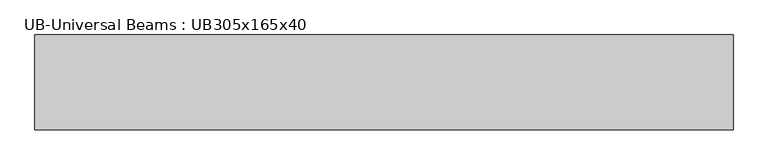
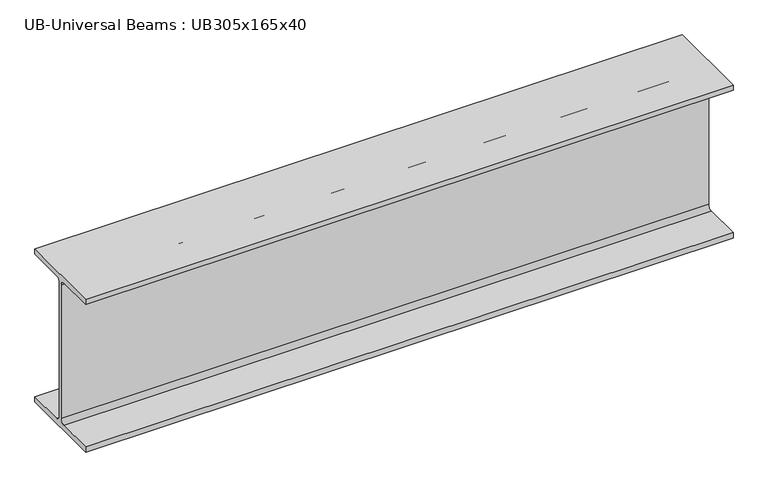
"""IFC4 building model written with IfcOpenShell, lengths in millimetres: beam geometry, UB-Universal Beams : UB305x165x40."""

from ifc_helpers import new_model, si_unit, point, frame, frame_2d, origin, place, context, project, spatial, polyline, circle_curve, trimmed, segment, composite_curve, outline, extrude, source, transform, mapped, element, save


def ub_universal_beams_ub305x165x40_babad7d3(model_context):
    return source(origin(), model_context, "Body", "SweptSolid", [
        extrude(outline(composite_curve([segment(polyline([(82.5, -141.5), (82.5, -151.7), (-82.5, -151.7), (-82.5, -141.5), (-11.9, -141.5)]), True, "CONTINUOUS"), segment(trimmed(circle_curve(frame_2d((-11.9, -132.6)), 8.9), [point((-11.9, -141.5))], [point((-3.0, -132.6))], True, "CARTESIAN"), True, "CONTINUOUS"), segment(polyline([(-3.0, -132.6), (-3.0, 132.6)]), True, "CONTINUOUS"), segment(trimmed(circle_curve(frame_2d((-11.9, 132.6)), 8.9), [point((-3.0, 132.6))], [point((-11.9, 141.5))], True, "CARTESIAN"), True, "CONTINUOUS"), segment(polyline([(-11.9, 141.5), (-82.5, 141.5), (-82.5, 151.7), (82.5, 151.7), (82.5, 141.5), (11.9, 141.5)]), True, "CONTINUOUS"), segment(trimmed(circle_curve(frame_2d((11.9, 132.6)), 8.9), [point((11.9, 141.5))], [point((3.0, 132.6))], True, "CARTESIAN"), True, "CONTINUOUS"), segment(polyline([(3.0, 132.6), (3.0, -132.6)]), True, "CONTINUOUS"), segment(trimmed(circle_curve(frame_2d((11.9, -132.6)), 8.9), [point((3.0, -132.6))], [point((11.9, -141.5))], True, "CARTESIAN"), True, "CONTINUOUS"), segment(polyline([(11.9, -141.5), (82.5, -141.5)]), True, "CONTINUOUS")], self_intersect=False)), frame((-824.1, 0.0, 0.0), z_axis=(1.0, 0.0, 0.0), x_axis=(0.0, 1.0, 0.0)), (0.0, 0.0, 1.0), 1215.8),
    ])


if __name__ == "__main__":
    model = new_model("IFC4")
    model_context = context("Model", 3, world=origin())
    ifc_project = project(units=[si_unit("LENGTHUNIT", "METRE", prefix="MILLI")], contexts=[model_context])
    site = spatial("IfcSite", under=ifc_project)
    building = spatial("IfcBuilding", under=site)
    placement = place(None, origin())
    ub_universal_beams_ub305x165x40_shape = ub_universal_beams_ub305x165x40_babad7d3(model_context)
    element("IfcBeam", 1, ObjectType="UB-Universal Beams : UB305x165x40", at=placement, inside=building, context=model_context, shape_type="MappedRepresentation", body=[
        mapped(ub_universal_beams_ub305x165x40_shape, transform((0.0, 0.0, 0.0), x_axis=(1.0, 0.0, 0.0), y_axis=(0.0, 1.0, 0.0), z_axis=(0.0, 0.0, 1.0))),
    ])
    save(model, "model.ifc")

# Revit data of these elements
# Type "UB-Universal Beams : UB305x165x40"
#   Section Name Key = "UB305X165X40"
#   Width = 16.5 cm
#   Web Thickness = 0.6 cm
#   Web Fillet = 0.89 cm
#   Warping Constant = 164000.0 cm⁶
#   Torsional Moment of Inertia = 14.70 cm⁴
#   Section Area = 51.3 cm²
#   Plastic Modulus weak axis = 142.0 cm³
#   Plastic Modulus strong axis = 623.0 cm³
#   Nominal Weight = 40.2999 kgf/m
#   Moment of Inertia weak axis = 764.00 cm⁴
#   Moment of Inertia strong axis = 8503.00 cm⁴
#   Height = 30.34 cm
#   Flange Thickness = 1.02 cm
#   Elastic Modulus weak axis = 92.6 cm³
#   Elastic Modulus strong axis = 560.0 cm³
#   Centroid Vertical = 15.17 cm
#   Centroid Horizontal = 8.25 cm
#   Bolt Spacing = 9.0 cm
#   Length [instance default] = 1500 mm
#   Structural Material [instance default] = Metal - Steel 43-275
#   Type Comments = ""
#   Assembly Code = ""
# Element 1 (IfcBeam, "UB-Universal Beams : UB305x165x40")
#   Materials on its faces: "Metal - Steel 43-275"
# Materials
#   "Metal - Steel 43-275": class "Metal", colour RGB 247 247 247, transparency 0, Cost = 0
